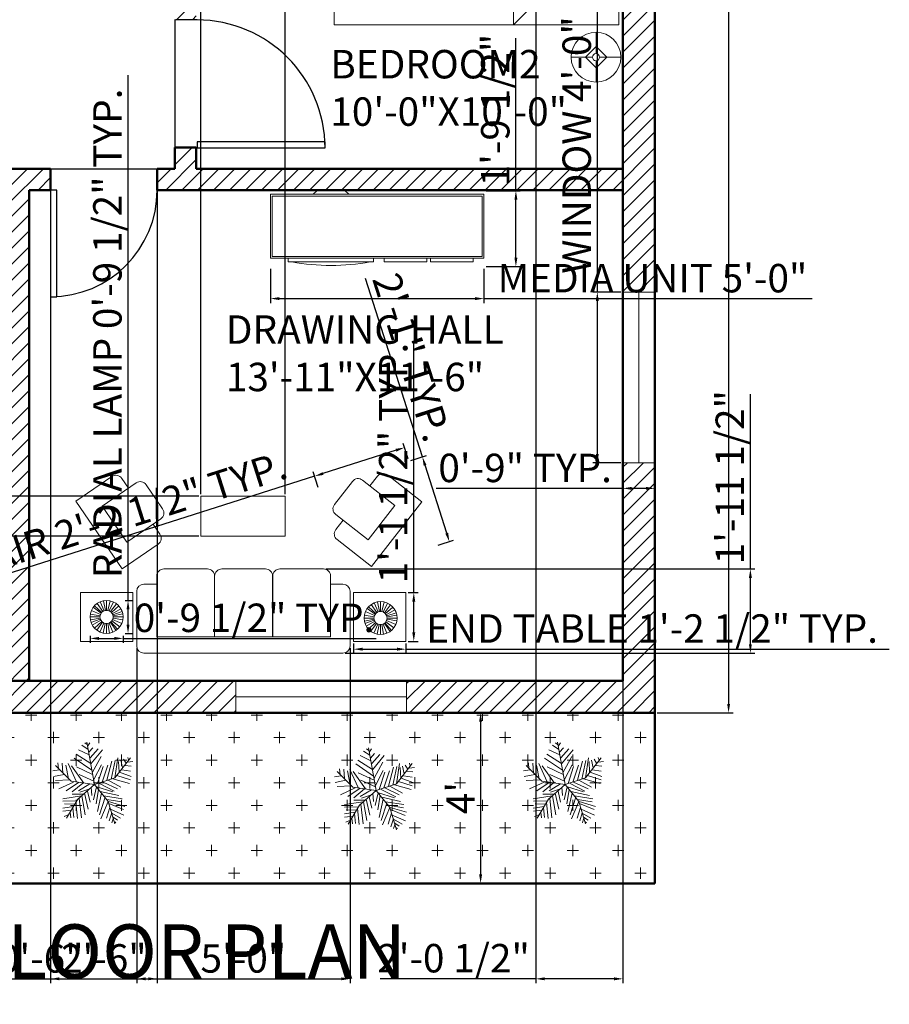
# Model space of a CAD drawing. Units: inches. Extents: x 1188 to 1681, y 1982 to 2608.
# Tile 2 of 4: x 1389 to 1634, y 1982 to 2259. Entities that reach past the tile are written whole.
import ezdxf

# ---------------------------------------------------------------- set-up
doc = ezdxf.new("R2010")
doc.units = ezdxf.units.IN
for name, color, linetype, lineweight in [('A-ANNO-DIMS', 2, 'Continuous', 18), ('A-ANNO-TEXT', 7, 'Continuous', 25), ('A-AREA-IDEN', 7, 'Continuous', 18), ('A-DOOR', 4, 'Continuous', 25), ('A-FURN', 8, 'Continuous', 18), ('A-GLAZ', 4, 'Continuous', 20), ('A-WALL', 7, 'Continuous', 50), ('A-WALL-PATT', 8, 'Continuous', 13)]:
    doc.layers.add(name, color=color, linetype=linetype, lineweight=lineweight)
doc.layers.add('L-PLNT', color=116, linetype='Continuous', lineweight=18, true_color=0x136734)
doc.layers.add('L-PLNT-PATT', color=116, linetype='Continuous', lineweight=13, true_color=0x136734)
doc.styles.get("Standard").update_dxf_attribs({"font": 'arial.ttf'})
doc.dimstyles.new('ISO-25', dxfattribs={"dimtxt": 8, "dimasz": 2.5, "dimexe": 1.25, "dimexo": 0.625, "dimtad": 1, "dimdec": 1, "dimlunit": 4, "dimtxsty": 'Standard', "dimcen": 2.5, "dimadec": 0, "dimazin": 0, "dimtfac": 1, "dimtdec": 1, "dimtmove": 0, "dimatfit": 3, "dimfxl": 1, "dimarcsym": 0})

# ---------------------------------------------------------------- blocks, each defined once
blk = doc.blocks.new('*U4')
for p, q in [((0, 0), (0, -6)), ((-36, 0), (-36, -6))]:
    blk.add_line(p, q)
blk.add_lwpolyline([(0, 0), (0, 36), (-1.75, 36), (-1.75, 0)], close=True)
blk.add_arc((0, 0), 36, 90, 180)
blk = doc.blocks.new('*U3')
for p, q in [((0, 0), (0, 6)), ((30, 0), (30, 6))]:
    blk.add_line(p, q)
blk.add_lwpolyline([(0, 0), (0, -30), (1.75, -30), (1.75, 0)], close=True)
blk.add_arc((0, 0), 30, 270, 0)
blk = doc.blocks.new('Entertainment Center')
for p, q in [((-4, 0), (-5, -1)), ((4, 0), (-4, 0)), ((5, -1), (4, 0)), ((-17, -19), (-17, -1)), ((-17, -1), (43, -1)), ((-16.5, -18.5), (-16.5, -1.5)), ((-16.5, -1.5), (42.5, -1.5)), ((42.5, -1.5), (42.5, -18.5)), ((43, -1), (43, -19)), ((43, -19), (-17, -19)), ((42.5, -18.5), (-16.5, -18.5)), ((-12, -20), (-12, -19)), ((12, -19), (12, -20)), ((15, -20), (15, -19)), ((27, -19), (27, -20)), ((28, -20), (28, -19)), ((40, -19), (40, -20)), ((12, -20), (-12, -20)), ((27, -20), (15, -20)), ((40, -20), (28, -20))]:
    blk.add_line(p, q)
blk.add_arc((0, 40), 61, 259.6111, 280.3889)
blk = doc.blocks.new('Lamp - Table')
for p, q in [((0, 7), (0, 1)), ((0, 3), (-3, 0)), ((3, 0), (0, 3)), ((-1, 0), (-7, 0)), ((-3, 0), (0, -3)), ((0, -3), (3, 0)), ((1, 0), (7, 0)), ((0, -1), (0, -7))]:
    blk.add_line(p, q)
for radius in [7, 1]:
    blk.add_circle((0, 0), radius)
blk = doc.blocks.new('Bed - Queen')
for p, q in [((0, -80.00003), (0, 0)), ((0, 0), (59.99999, 0)), ((59.99999, 0), (59.99999, -80.00003)), ((7.99999, -1.2), (28.79998, -1.2)), ((7.99999, -14.4), (7.99999, -1.2)), ((28.79998, -1.2), (28.79998, -14.4)), ((31.19999, -1.2), (51.99999, -1.2)), ((31.19999, -14.4), (31.19999, -1.2)), ((51.99999, -1.2), (51.99999, -16.4)), ((0, -14.4), (44.8, -14.4)), ((59.99999, -29.6), (44.8, -14.4)), ((44.8, -14.4), (44.8, -29.6)), ((51.99999, -16.4), (46.79936, -16.4)), ((44.8, -16.8), (0, -16.8)), ((44.8, -29.6), (59.99999, -29.6)), ((59.99999, -80.00003), (0, -80.00003))]:
    blk.add_line(p, q)
blk = doc.blocks.new('*U12')
for p, q in [((-8.737, 47.138), (-17.069, 52.711)), ((-10.186, 53.64), (-13.084, 55.962)), ((0, 0), (-10.5, 57)), ((-9.099, 51.782), (-6.563, 55.962)), ((-5.114, 28.097), (-24.676, 40.636)), ((-7.288, 39.707), (-21.778, 46.673)), ((-7.65, 43.423), (-2.578, 49.46)), ((-5.839, 35.992), (4.667, 48.067)), ((-5.114, 27.632), (10.463, 46.673)), ((-48.585, 21.131), (-49.309, 29.026)), ((-43.513, 28.561), (-42.427, 15.558)), ((-35.544, 28.097), (-24.314, 3.947)), ((-3.665, 19.273), (-27.574, 35.527)), ((-2.941, 16.486), (8.652, 37.85)), ((-1.129, 6.734), (9.014, 26.704)), ((16.259, 5.805), (23.142, 31.348)), ((22.055, 7.198), (27.489, 32.277)), ((27, 9), (48, 36)), ((27.127, 9.056), (31.112, 35.992)), ((31.836, 30.883), (32.561, 16.486)), ((35.096, 32.741), (37.27, 22.524)), ((38.719, 34.134), (41.979, 28.561)), ((43.791, 29.954), (51.036, 30.883)), ((44.153, 36.456), (45.239, 32.741)), ((-47.498, 19.737), (-55.83, 18.344)), ((-40.615, 13.7), (-55.105, 10.913)), ((-31.5, 4.5), (-52.5, 25.5)), ((-38.442, 26.239), (-34.819, 7.663)), ((-14.533, 2.09), (-30.834, 25.31)), ((-24.314, 23.917), (-2.941, 13.7)), ((-20.691, 13.7), (-1.129, 4.876)), ((3.942, 1.625), (11.187, 24.381)), ((10.101, 3.483), (17.708, 26.239)), ((33.285, 16.486), (48.862, 10.913)), ((36.183, 19.737), (48.137, 17.88)), ((40.53, 25.775), (48.862, 24.846)), ((-33.37, 6.269), (-52.207, 5.34)), ((-28.299, 3.483), (-47.86, -5.805)), ((-21.416, 3.018), (-38.079, -8.128)), ((0, 0), (-31.5, 4.5)), ((-15.982, 2.09), (-30.11, -9.521)), ((0, 0), (-22.5, -19.5)), ((-6.563, 1.161), (-21.416, -8.128)), ((0, 0), (27, 9)), ((0, 0), (18, -22.5)), ((6.478, 1.625), (26.04, -8.592)), ((11.187, 3.483), (30.749, -5.805)), ((18.07, 5.805), (35.096, -3.483)), ((24.229, 7.663), (46.688, 1.625)), ((29.662, 12.307), (48.137, 6.269)), ((-15.257, -12.772), (-30.11, -12.772)), ((-6.563, -5.805), (-19.967, -9.985)), ((-13.446, -11.378), (-8.737, -32.741)), ((-9.461, -8.592), (-6.201, -23.453)), ((-4.752, -3.483), (-3.665, -14.629)), ((2.493, -3.019), (-1.491, -20.202)), ((1.769, -2.555), (24.229, -9.521)), ((5.029, -6.27), (2.131, -25.775)), ((9.014, -11.378), (3.58, -35.992)), ((7.565, -9.056), (32.198, -14.629)), ((-17.431, -15.094), (-42.789, -18.809)), ((-24.314, -21.596), (-42.427, -22.06)), ((-26.849, -26.24), (-40.253, -25.775)), ((-22.5, -19.5), (-37.5, -45)), ((-25.038, -23.918), (-22.865, -45.281)), ((-20.691, -18.345), (-17.793, -44.352)), ((-17.069, -15.094), (-12.721, -40.172)), ((14.085, -16.951), (6.478, -40.172)), ((18.07, -22.524), (8.289, -45.745)), ((12.274, -15.094), (36.907, -18.809)), ((16.259, -19.738), (36.183, -22.989)), ((18, -22.5), (27, -52.5)), ((18.433, -22.524), (40.53, -29.026)), ((19.157, -25.311), (38.719, -33.206)), ((-28.299, -29.026), (-42.789, -31.348)), ((-30.834, -34.135), (-42.427, -35.528)), ((-32.646, -36.921), (-31.921, -44.352)), ((-29.023, -30.884), (-27.936, -43.887)), ((20.244, -30.419), (15.897, -44.816)), ((22.78, -37.85), (19.519, -48.532)), ((21.331, -32.741), (39.081, -40.636)), ((22.78, -38.314), (34.372, -44.816)), ((-34.457, -39.708), (-40.978, -42.494)), ((24.591, -45.745), (23.142, -50.854)), ((24.591, -43.423), (30.749, -47.603)), ((26.764, -49.925), (28.213, -50.854))]:
    blk.add_line(p, q)
blk = doc.blocks.new('*D13')
at = {"layer": 'A-ANNO-DIMS', "color": 0, "lineweight": -2, "transparency": 16777216}
for p, q in [((1568.34, 2496.41), (1589.68, 2496.41)), ((1588.43, 2493.91), (1588.43, 2066.91)), ((1568.34, 2064.41), (1589.68, 2064.41))]:
    blk.add_line(p, q, dxfattribs=at)
at = {"layer": 'A-ANNO-DIMS', "color": 0, "transparency": 16777216}
for points in [[(1588.02, 2493.91), (1588.85, 2493.91), (1588.43, 2496.41)], [(1588.02, 2066.91), (1588.85, 2066.91), (1588.43, 2064.41)]]:
    blk.add_solid(points, dxfattribs=at)
at = {"layer": 'Defpoints', "color": 0, "transparency": 16777216}
for p in [(1567.72, 2496.41), (1567.72, 2064.41), (1588.43, 2064.41)]:
    blk.add_point(p, dxfattribs=at)
at = {"layer": 'A-ANNO-DIMS', "color": 0, "transparency": 16777216, "insert": (1583.72, 2280.41), "char_height": 8, "attachment_point": 5, "rotation": 90}
blk.add_mtext("36'", dxfattribs=at)
blk = doc.blocks.new('*D15')
at = {"layer": 'A-ANNO-DIMS', "color": 0, "lineweight": -2, "transparency": 16777216}
for p, q in [((1512.39, 2064.41), (1519.94, 2064.41)), ((1518.69, 2061.91), (1518.69, 2018.91)), ((1512.39, 2016.41), (1519.94, 2016.41))]:
    blk.add_line(p, q, dxfattribs=at)
at = {"layer": 'A-ANNO-DIMS', "color": 0, "transparency": 16777216}
for points in [[(1518.27, 2061.91), (1519.1, 2061.91), (1518.69, 2064.41)], [(1518.27, 2018.91), (1519.1, 2018.91), (1518.69, 2016.41)]]:
    blk.add_solid(points, dxfattribs=at)
at = {"layer": 'Defpoints', "color": 0, "transparency": 16777216}
for p in [(1511.77, 2064.41), (1511.77, 2016.41), (1518.69, 2016.41)]:
    blk.add_point(p, dxfattribs=at)
at = {"layer": 'A-ANNO-DIMS', "color": 0, "transparency": 16777216, "insert": (1514.06, 2040.41), "char_height": 8, "attachment_point": 5, "rotation": 90}
blk.add_mtext("4'", dxfattribs=at)
blk = doc.blocks.new('WIN-48IN')
for p, q in [((0, 9), (0, 0)), ((48, 0), (48, 9)), ((48, 9), (48, 4.5)), ((48, 4.5), (0, 4.5)), ((0, 0), (48, 0))]:
    blk.add_line(p, q)
blk = doc.blocks.new('CHAIR-LOUNGE')
for p, q in [((10.14, 25.95), (0, 18.99)), ((14.8, 22.68), (12.92, 25.43)), ((0, 18.99), (13.03, 0)), ((23.68, 9.73), (21.74, 12.56)), ((13.03, 0), (23.17, 6.95))]:
    blk.add_line(p, q)
blk.add_lwpolyline([(16.97, 24.17), (7.41, 17.62), (14.35, 7.5), (23.91, 14.05, 0.414214), (24.43, 16.83), (19.75, 23.65, 0.414214)], format="xyb", close=True)
for centre, start, end in [((11.27, 24.3), 34.4415, 124.4415), ((22.03, 8.6), 304.4415, 34.4415)]:
    blk.add_arc(centre, 2, start, end)
blk = doc.blocks.new('LAMP-RADIAL-TABLE')
for p, q in [((1.97, 8.43), (3.57, 6.16)), ((3.57, 6.16), (1.97, 8.43)), ((3.92, 6.36), (2.86, 8.92)), ((2.86, 8.92), (3.92, 6.36)), ((4.31, 6.47), (3.81, 9.2)), ((3.81, 9.2), (4.31, 6.47)), ((4.64, 6.5), (4.64, 9.28)), ((5.01, 6.46), (5.61, 9.18)), ((5.61, 9.18), (5.03, 6.46)), ((5.41, 6.34), (6.55, 8.87)), ((5.75, 6.14), (7.4, 8.37)), ((7.4, 8.37), (5.75, 6.14)), ((2.93, 5.37), (0.37, 6.46)), ((0.89, 7.37), (3.13, 5.74)), ((3.13, 5.74), (0.89, 7.37)), ((3.28, 5.91), (1.25, 7.8)), ((6.03, 5.88), (8.1, 7.73)), ((6.26, 5.56), (8.67, 6.93)), ((8.67, 6.93), (6.26, 5.56)), ((6.4, 5.24), (9.03, 6.15)), ((2.78, 4.64), (0, 4.64)), ((0.07, 5.42), (2.8, 4.95)), ((2.8, 4.95), (0.07, 5.42)), ((2.8, 4.34), (0.08, 3.8)), ((0.08, 3.8), (2.81, 4.3)), ((2.88, 4.04), (0.25, 3.13)), ((0.25, 3.13), (2.88, 4.04)), ((0.6, 2.35), (3.02, 3.72)), ((3.02, 3.72), (0.6, 2.35)), ((3.26, 3.39), (1.21, 1.52)), ((1.88, 0.91), (3.52, 3.15)), ((3.53, 3.14), (1.88, 0.91)), ((3.87, 2.94), (2.73, 0.41)), ((3.67, 0.1), (4.23, 2.82)), ((4.25, 2.82), (3.67, 0.1)), ((4.64, 2.78), (4.64, 0)), ((5.47, 0.07), (4.97, 2.81)), ((4.97, 2.81), (5.47, 0.07)), ((5.36, 2.92), (6.42, 0.36)), ((7.31, 0.85), (5.71, 3.12)), ((5.71, 3.12), (7.31, 0.85)), ((5.88, 3.25), (7.72, 1.17)), ((6.14, 3.54), (8.39, 1.91)), ((8.39, 1.91), (6.14, 3.54)), ((6.35, 3.91), (8.91, 2.82)), ((8.91, 2.82), (6.35, 3.91)), ((6.47, 4.98), (9.2, 5.48)), ((9.21, 3.85), (6.47, 4.32)), ((6.47, 4.32), (9.21, 3.85)), ((9.28, 4.64), (6.5, 4.64))]:
    blk.add_line(p, q)
for radius in [4.64, 1.86]:
    blk.add_circle((4.64, 4.64), radius)
blk = doc.blocks.new('TABLE-END')
blk.add_lwpolyline([(14.72, 0), (0, 0), (0, 13.7), (14.72, 13.7)], close=True)
blk = doc.blocks.new('*D26')
at = {"layer": 'A-ANNO-DIMS', "color": 0, "lineweight": -2, "transparency": 16777216}
for p, q in [((1551.52, 2182.72), (1551.52, 2287.7)), ((1558.09, 2182.72), (1550.27, 2182.72)), ((1551.52, 2137.22), (1551.52, 2180.22)), ((1558.09, 2134.72), (1550.27, 2134.72))]:
    blk.add_line(p, q, dxfattribs=at)
at = {"layer": 'A-ANNO-DIMS', "color": 0, "transparency": 16777216}
for points in [[(1551.1, 2180.22), (1551.93, 2180.22), (1551.52, 2182.72)], [(1551.1, 2137.22), (1551.93, 2137.22), (1551.52, 2134.72)]]:
    blk.add_solid(points, dxfattribs=at)
at = {"layer": 'Defpoints', "color": 0, "transparency": 16777216}
for p in [(1551.52, 2182.72), (1558.72, 2182.72), (1558.72, 2134.72)]:
    blk.add_point(p, dxfattribs=at)
at = {"layer": 'A-ANNO-DIMS', "color": 0, "transparency": 16777216, "insert": (1546.75, 2236.46), "char_height": 8, "attachment_point": 5, "rotation": 90}
blk.add_mtext('WINDOW 4\'-0" TYP.', dxfattribs=at)
blk = doc.blocks.new('*D27')
at = {"layer": 'A-ANNO-DIMS', "color": 0, "lineweight": -2, "transparency": 16777216}
for p, q in [((1558.72, 2134.09), (1558.72, 2126.27)), ((1567.72, 2134.09), (1567.72, 2126.27)), ((1558.72, 2127.52), (1506.2, 2127.52)), ((1565.22, 2127.52), (1561.22, 2127.52))]:
    blk.add_line(p, q, dxfattribs=at)
at = {"layer": 'A-ANNO-DIMS', "color": 0, "transparency": 16777216}
for points in [[(1561.22, 2127.93), (1561.22, 2127.1), (1558.72, 2127.52)], [(1565.22, 2127.93), (1565.22, 2127.1), (1567.72, 2127.52)]]:
    blk.add_solid(points, dxfattribs=at)
at = {"layer": 'Defpoints', "color": 0, "transparency": 16777216}
for p in [(1558.72, 2134.72), (1567.72, 2134.72), (1558.72, 2127.52)]:
    blk.add_point(p, dxfattribs=at)
at = {"layer": 'A-ANNO-DIMS', "color": 0, "transparency": 16777216, "insert": (1531.21, 2132.23), "char_height": 8, "attachment_point": 5}
blk.add_mtext('0\'-9" TYP.', dxfattribs=at)
blk = doc.blocks.new('*D30')
at = {"layer": 'A-ANNO-DIMS', "color": 0, "lineweight": -2, "transparency": 16777216}
for p, q in [((1494.92, 2138.23), (1474.36, 2131.69)), ((1498.32, 2135.79), (1496.92, 2140.18)), ((1471.98, 2130.93), (1320.5, 2082.67)), ((1473, 2127.73), (1471.6, 2132.12))]:
    blk.add_line(p, q, dxfattribs=at)
at = {"layer": 'A-ANNO-DIMS', "color": 0, "transparency": 16777216}
for points in [[(1494.79, 2138.63), (1495.04, 2137.84), (1497.3, 2138.99)], [(1474.24, 2132.08), (1474.49, 2131.29), (1471.98, 2130.93)]]:
    blk.add_solid(points, dxfattribs=at)
at = {"layer": 'Defpoints', "color": 0, "transparency": 16777216}
for p in [(1498.51, 2135.2), (1471.98, 2130.93), (1473.19, 2127.13)]:
    blk.add_point(p, dxfattribs=at)
at = {"layer": 'A-ANNO-DIMS', "color": 0, "transparency": 16777216, "insert": (1393.6, 2110.96), "char_height": 8, "attachment_point": 5, "rotation": 17.6695}
blk.add_mtext('LOUNGE CHAIR 2\'-2 1/2" TYP.', dxfattribs=at)
blk = doc.blocks.new('*D31')
at = {"layer": 'A-ANNO-DIMS', "color": 0, "lineweight": -2, "transparency": 16777216}
for p, q in [((1502.31, 2136.41), (1486.33, 2186.57)), ((1499.1, 2135.39), (1503.5, 2136.79)), ((1509.15, 2114.91), (1503.07, 2134.02)), ((1506.71, 2111.51), (1511.1, 2112.91))]:
    blk.add_line(p, q, dxfattribs=at)
at = {"layer": 'A-ANNO-DIMS', "color": 0, "transparency": 16777216}
for points in [[(1503.46, 2134.15), (1502.67, 2133.9), (1502.31, 2136.41)], [(1509.55, 2115.04), (1508.76, 2114.79), (1509.91, 2112.53)]]:
    blk.add_solid(points, dxfattribs=at)
at = {"layer": 'Defpoints', "color": 0, "transparency": 16777216}
for p in [(1502.31, 2136.41), (1498.51, 2135.2), (1506.11, 2111.32)]:
    blk.add_point(p, dxfattribs=at)
at = {"layer": 'A-ANNO-DIMS', "color": 0, "transparency": 16777216, "insert": (1498.36, 2164.09), "char_height": 8, "attachment_point": 5, "rotation": 287.6695}
blk.add_mtext('2\'-1" TYP.', dxfattribs=at)
blk = doc.blocks.new('*D32')
at = {"layer": 'A-ANNO-DIMS', "color": 0, "lineweight": -2, "transparency": 16777216}
for p, q in [((1419.52, 2095.98), (1419.52, 2243.74)), ((1418.76, 2095.98), (1420.77, 2095.98)), ((1419.52, 2089.2), (1419.52, 2093.48)), ((1418.76, 2086.7), (1420.77, 2086.7))]:
    blk.add_line(p, q, dxfattribs=at)
at = {"layer": 'A-ANNO-DIMS', "color": 0, "transparency": 16777216}
for points in [[(1419.11, 2093.48), (1419.94, 2093.48), (1419.52, 2095.98)], [(1419.11, 2089.2), (1419.94, 2089.2), (1419.52, 2086.7)]]:
    blk.add_solid(points, dxfattribs=at)
at = {"layer": 'Defpoints', "color": 0, "transparency": 16777216}
for p in [(1418.13, 2095.98), (1419.52, 2095.98), (1418.13, 2086.7)]:
    blk.add_point(p, dxfattribs=at)
at = {"layer": 'A-ANNO-DIMS', "color": 0, "transparency": 16777216, "insert": (1414.76, 2171.11), "char_height": 8, "attachment_point": 5, "rotation": 90}
blk.add_mtext('RADIAL LAMP 0\'-9 1/2" TYP.', dxfattribs=at)
blk = doc.blocks.new('*D33')
at = {"layer": 'A-ANNO-DIMS', "color": 0, "lineweight": -2, "transparency": 16777216}
for p, q in [((1408.85, 2086.08), (1408.85, 2084.06)), ((1418.13, 2086.08), (1418.13, 2084.06)), ((1411.35, 2085.31), (1415.63, 2085.31)), ((1418.13, 2085.31), (1489.29, 2085.31))]:
    blk.add_line(p, q, dxfattribs=at)
at = {"layer": 'A-ANNO-DIMS', "color": 0, "transparency": 16777216}
for points in [[(1411.35, 2085.73), (1411.35, 2084.89), (1408.85, 2085.31)], [(1415.63, 2085.73), (1415.63, 2084.89), (1418.13, 2085.31)]]:
    blk.add_solid(points, dxfattribs=at)
at = {"layer": 'Defpoints', "color": 0, "transparency": 16777216}
for p in [(1408.85, 2086.7), (1418.13, 2086.7), (1418.13, 2085.31)]:
    blk.add_point(p, dxfattribs=at)
at = {"layer": 'A-ANNO-DIMS', "color": 0, "transparency": 16777216, "insert": (1454.96, 2090.07), "char_height": 8, "attachment_point": 5}
blk.add_mtext('0\'-9 1/2" TYP.', dxfattribs=at)
blk = doc.blocks.new('*D34')
at = {"layer": 'A-ANNO-DIMS', "color": 0, "lineweight": -2, "transparency": 16777216}
for p, q in [((1482.97, 2083.87), (1482.97, 2081.03)), ((1497.69, 2083.87), (1497.69, 2081.03)), ((1485.47, 2082.28), (1495.19, 2082.28)), ((1497.69, 2082.28), (1633.64, 2082.28))]:
    blk.add_line(p, q, dxfattribs=at)
at = {"layer": 'A-ANNO-DIMS', "color": 0, "transparency": 16777216}
for points in [[(1485.47, 2082.7), (1485.47, 2081.87), (1482.97, 2082.28)], [(1495.19, 2082.7), (1495.19, 2081.87), (1497.69, 2082.28)]]:
    blk.add_solid(points, dxfattribs=at)
at = {"layer": 'Defpoints', "color": 0, "transparency": 16777216}
for p in [(1482.97, 2084.49), (1497.69, 2084.49), (1497.69, 2082.28)]:
    blk.add_point(p, dxfattribs=at)
at = {"layer": 'A-ANNO-DIMS', "color": 0, "transparency": 16777216, "insert": (1566.91, 2087.05), "char_height": 8, "attachment_point": 5}
blk.add_mtext('END TABLE 1\'-2 1/2" TYP.', dxfattribs=at)
blk = doc.blocks.new('*D35')
at = {"layer": 'A-ANNO-DIMS', "color": 0, "lineweight": -2, "transparency": 16777216}
for p, q in [((1499.9, 2098.19), (1499.9, 2168.6)), ((1498.31, 2098.19), (1501.15, 2098.19)), ((1499.9, 2086.99), (1499.9, 2095.69)), ((1498.31, 2084.49), (1501.15, 2084.49))]:
    blk.add_line(p, q, dxfattribs=at)
at = {"layer": 'A-ANNO-DIMS', "color": 0, "transparency": 16777216}
for points in [[(1499.48, 2095.69), (1500.31, 2095.69), (1499.9, 2098.19)], [(1499.48, 2086.99), (1500.31, 2086.99), (1499.9, 2084.49)]]:
    blk.add_solid(points, dxfattribs=at)
at = {"layer": 'Defpoints', "color": 0, "transparency": 16777216}
for p in [(1497.69, 2098.19), (1499.9, 2098.19), (1497.69, 2084.49)]:
    blk.add_point(p, dxfattribs=at)
at = {"layer": 'A-ANNO-DIMS', "color": 0, "transparency": 16777216, "insert": (1495.14, 2134.64), "char_height": 8, "attachment_point": 5, "rotation": 90}
blk.add_mtext('1\'-1 1/2" TYP.', dxfattribs=at)
blk = doc.blocks.new('*D40')
at = {"layer": 'A-ANNO-DIMS', "color": 0, "lineweight": -2, "transparency": 16777216}
for p, q in [((1459.61, 2189.27), (1459.61, 2179.64)), ((1519.61, 2189.27), (1519.61, 2179.64)), ((1462.11, 2180.89), (1517.11, 2180.89)), ((1519.61, 2180.89), (1611.94, 2180.89))]:
    blk.add_line(p, q, dxfattribs=at)
at = {"layer": 'A-ANNO-DIMS', "color": 0, "transparency": 16777216}
for points in [[(1462.11, 2181.31), (1462.11, 2180.47), (1459.61, 2180.89)], [(1517.11, 2181.31), (1517.11, 2180.47), (1519.61, 2180.89)]]:
    blk.add_solid(points, dxfattribs=at)
at = {"layer": 'Defpoints', "color": 0, "transparency": 16777216}
for p in [(1459.61, 2189.89), (1519.61, 2189.89), (1519.61, 2180.89)]:
    blk.add_point(p, dxfattribs=at)
at = {"layer": 'A-ANNO-DIMS', "color": 0, "transparency": 16777216, "insert": (1567.03, 2185.6), "char_height": 8, "attachment_point": 5}
blk.add_mtext('MEDIA UNIT 5\'-0"', dxfattribs=at)
blk = doc.blocks.new('*D41')
at = {"layer": 'A-ANNO-DIMS', "color": 0, "lineweight": -2, "transparency": 16777216}
for p, q in [((1528.61, 2211.22), (1528.61, 2254.13)), ((1520.24, 2211.22), (1529.86, 2211.22)), ((1528.61, 2192.39), (1528.61, 2208.72)), ((1520.24, 2189.89), (1529.86, 2189.89))]:
    blk.add_line(p, q, dxfattribs=at)
at = {"layer": 'A-ANNO-DIMS', "color": 0, "transparency": 16777216}
for points in [[(1528.2, 2208.72), (1529.03, 2208.72), (1528.61, 2211.22)], [(1528.2, 2192.39), (1529.03, 2192.39), (1528.61, 2189.89)]]:
    blk.add_solid(points, dxfattribs=at)
at = {"layer": 'Defpoints', "color": 0, "transparency": 16777216}
for p in [(1519.61, 2211.22), (1528.61, 2211.22), (1519.61, 2189.89)]:
    blk.add_point(p, dxfattribs=at)
at = {"layer": 'A-ANNO-DIMS', "color": 0, "transparency": 16777216, "insert": (1523.85, 2233.93), "char_height": 8, "attachment_point": 5, "rotation": 90}
blk.add_mtext('1\'-9 1/2"', dxfattribs=at)
blk = doc.blocks.new('*D48')
at = {"layer": 'A-ANNO-DIMS', "color": 0, "lineweight": -2, "transparency": 16777216}
for p, q in [((1397.72, 2216.79), (1397.72, 1988.31)), ((1427.72, 2216.79), (1427.72, 1988.31)), ((1400.22, 1989.56), (1425.22, 1989.56))]:
    blk.add_line(p, q, dxfattribs=at)
at = {"layer": 'A-ANNO-DIMS', "color": 0, "transparency": 16777216}
for points in [[(1400.22, 1989.98), (1400.22, 1989.15), (1397.72, 1989.56)], [(1425.22, 1989.98), (1425.22, 1989.15), (1427.72, 1989.56)]]:
    blk.add_solid(points, dxfattribs=at)
at = {"layer": 'Defpoints', "color": 0, "transparency": 16777216}
for p in [(1397.72, 2217.41), (1427.72, 2217.41), (1427.72, 1989.56)]:
    blk.add_point(p, dxfattribs=at)
at = {"layer": 'A-ANNO-DIMS', "color": 0, "transparency": 16777216, "insert": (1412.72, 1994.27), "char_height": 8, "attachment_point": 5}
blk.add_mtext('2\'-6"', dxfattribs=at)
blk = doc.blocks.new('*D50')
at = {"layer": 'A-ANNO-DIMS', "color": 0, "lineweight": -2, "transparency": 16777216}
for p, q in [((1372.72, 2342.79), (1372.72, 1988.31)), ((1378.72, 2336.79), (1378.72, 1988.31)), ((1370.22, 1989.56), (1367.72, 1989.56)), ((1372.72, 1989.56), (1378.72, 1989.56)), ((1381.22, 1989.56), (1406.23, 1989.56))]:
    blk.add_line(p, q, dxfattribs=at)
at = {"layer": 'A-ANNO-DIMS', "color": 0, "transparency": 16777216}
for points in [[(1370.22, 1989.98), (1370.22, 1989.15), (1372.72, 1989.56)], [(1381.22, 1989.98), (1381.22, 1989.15), (1378.72, 1989.56)]]:
    blk.add_solid(points, dxfattribs=at)
at = {"layer": 'Defpoints', "color": 0, "transparency": 16777216}
for p in [(1372.72, 2343.41), (1378.72, 2337.41), (1378.72, 1989.56)]:
    blk.add_point(p, dxfattribs=at)
at = {"layer": 'A-ANNO-DIMS', "color": 0, "transparency": 16777216, "insert": (1394.97, 1994.27), "char_height": 8, "attachment_point": 5}
blk.add_mtext('0\'-6"', dxfattribs=at)
blk = doc.blocks.new('*D52')
at = {"layer": 'A-ANNO-DIMS', "color": 0, "lineweight": -2, "transparency": 16777216}
for p, q in [((1534.2, 2391.18), (1534.2, 1988.31)), ((1558.72, 2391.18), (1558.72, 1988.31)), ((1534.2, 1989.56), (1490.41, 1989.56)), ((1556.22, 1989.56), (1536.7, 1989.56))]:
    blk.add_line(p, q, dxfattribs=at)
at = {"layer": 'A-ANNO-DIMS', "color": 0, "transparency": 16777216}
for points in [[(1536.7, 1989.98), (1536.7, 1989.15), (1534.2, 1989.56)], [(1556.22, 1989.98), (1556.22, 1989.15), (1558.72, 1989.56)]]:
    blk.add_solid(points, dxfattribs=at)
at = {"layer": 'Defpoints', "color": 0, "transparency": 16777216}
for p in [(1534.2, 2391.81), (1558.72, 2391.81), (1534.2, 1989.56)]:
    blk.add_point(p, dxfattribs=at)
at = {"layer": 'A-ANNO-DIMS', "color": 0, "transparency": 16777216, "insert": (1511.06, 1994.33), "char_height": 8, "attachment_point": 5}
blk.add_mtext('2\'-0 1/2"', dxfattribs=at)
blk = doc.blocks.new('*D57')
at = {"layer": 'A-ANNO-DIMS', "color": 0, "lineweight": -2, "transparency": 16777216}
for p, q in [((1440.02, 2125.93), (1440.02, 2524.51)), ((1442.52, 2523.26), (1461.18, 2523.26)), ((1463.68, 2125.93), (1463.68, 2524.51)), ((1463.68, 2523.26), (1512.8, 2523.26))]:
    blk.add_line(p, q, dxfattribs=at)
at = {"layer": 'A-ANNO-DIMS', "color": 0, "transparency": 16777216}
for points in [[(1442.52, 2523.68), (1442.52, 2522.85), (1440.02, 2523.26)], [(1461.18, 2523.68), (1461.18, 2522.85), (1463.68, 2523.26)]]:
    blk.add_solid(points, dxfattribs=at)
at = {"layer": 'Defpoints', "color": 0, "transparency": 16777216}
for p in [(1463.68, 2523.26), (1440.02, 2125.31), (1463.68, 2125.31)]:
    blk.add_point(p, dxfattribs=at)
at = {"layer": 'A-ANNO-DIMS', "color": 0, "transparency": 16777216, "insert": (1489.49, 2528.03), "char_height": 8, "attachment_point": 5}
blk.add_mtext('1\'-11 1/2"', dxfattribs=at)
blk = doc.blocks.new('*D58')
at = {"layer": 'A-ANNO-DIMS', "color": 0, "lineweight": -2, "transparency": 16777216}
for p, q in [((1204.87, 2125.31), (1204.87, 2175.18)), ((1439.4, 2125.31), (1203.62, 2125.31)), ((1204.87, 2116.54), (1204.87, 2122.81)), ((1439.4, 2114.04), (1203.62, 2114.04))]:
    blk.add_line(p, q, dxfattribs=at)
at = {"layer": 'A-ANNO-DIMS', "color": 0, "transparency": 16777216}
for points in [[(1204.45, 2122.81), (1205.28, 2122.81), (1204.87, 2125.31)], [(1204.45, 2116.54), (1205.28, 2116.54), (1204.87, 2114.04)]]:
    blk.add_solid(points, dxfattribs=at)
at = {"layer": 'Defpoints', "color": 0, "transparency": 16777216}
for p in [(1204.87, 2125.31), (1440.02, 2125.31), (1440.02, 2114.04)]:
    blk.add_point(p, dxfattribs=at)
at = {"layer": 'A-ANNO-DIMS', "color": 0, "transparency": 16777216, "insert": (1200.11, 2151.49), "char_height": 8, "attachment_point": 5, "rotation": 90}
blk.add_mtext('0\'-11 1/2"', dxfattribs=at)
blk = doc.blocks.new('*D59')
at = {"layer": 'A-ANNO-DIMS', "color": 0, "lineweight": -2, "transparency": 16777216}
for p, q in [((1421.97, 2082.56), (1421.97, 1988.31)), ((1481.97, 2082.56), (1481.97, 1988.31)), ((1424.47, 1989.56), (1479.47, 1989.56))]:
    blk.add_line(p, q, dxfattribs=at)
at = {"layer": 'A-ANNO-DIMS', "color": 0, "transparency": 16777216}
for points in [[(1424.47, 1989.98), (1424.47, 1989.15), (1421.97, 1989.56)], [(1479.47, 1989.98), (1479.47, 1989.15), (1481.97, 1989.56)]]:
    blk.add_solid(points, dxfattribs=at)
at = {"layer": 'Defpoints', "color": 0, "transparency": 16777216}
for p in [(1421.97, 2083.18), (1481.97, 2083.18), (1481.97, 1989.56)]:
    blk.add_point(p, dxfattribs=at)
at = {"layer": 'A-ANNO-DIMS', "color": 0, "transparency": 16777216, "insert": (1451.97, 1994.27), "char_height": 8, "attachment_point": 5}
blk.add_mtext('5\'-0"', dxfattribs=at)
blk = doc.blocks.new('*D60')
at = {"layer": 'A-ANNO-DIMS', "color": 0, "lineweight": -2, "transparency": 16777216}
for p, q in [((1594.57, 2104.85), (1594.57, 2153.97)), ((1475.13, 2104.85), (1595.82, 2104.85)), ((1594.57, 2083.68), (1594.57, 2102.35)), ((1480.59, 2081.18), (1595.82, 2081.18))]:
    blk.add_line(p, q, dxfattribs=at)
at = {"layer": 'A-ANNO-DIMS', "color": 0, "transparency": 16777216}
for points in [[(1594.15, 2102.35), (1594.98, 2102.35), (1594.57, 2104.85)], [(1594.15, 2083.68), (1594.98, 2083.68), (1594.57, 2081.18)]]:
    blk.add_solid(points, dxfattribs=at)
at = {"layer": 'Defpoints', "color": 0, "transparency": 16777216}
for p in [(1474.51, 2104.85), (1594.57, 2104.85), (1479.97, 2081.18)]:
    blk.add_point(p, dxfattribs=at)
at = {"layer": 'A-ANNO-DIMS', "color": 0, "transparency": 16777216, "insert": (1589.81, 2130.66), "char_height": 8, "attachment_point": 5, "rotation": 90}
blk.add_mtext('1\'-11 1/2"', dxfattribs=at)

msp = doc.modelspace()

# ---------------------------------------------------------------- hatches: boundary and pattern name
at = {"layer": 'A-WALL-PATT', "transparency": 33554559}
h = msp.add_hatch(dxfattribs=at)
h.set_pattern_fill('ANSI31', color=256)
h.paths.add_polyline_path([(1390.99, 2496.41), (1231.72, 2496.41), (1231.72, 2452.82), (1240.72, 2452.82), (1240.72, 2487.41), (1390.99, 2487.41)])
h.paths.add_polyline_path([(1469.3, 2496.41), (1426.99, 2496.41), (1426.99, 2491.91), (1426.99, 2487.41), (1469.3, 2487.41)])
h.paths.add_polyline_path([(1378.72, 2487.41), (1372.72, 2487.41), (1372.72, 2404.84), (1372.72, 2343.41), (1367.48, 2343.41), (1367.48, 2337.41), (1378.72, 2337.41), (1378.72, 2391.41), (1387.67, 2391.41), (1387.67, 2397.41), (1378.72, 2397.41)])
h.paths.add_polyline_path([(1438.72, 2487.41), (1432.72, 2487.41), (1432.72, 2397.41), (1420.72, 2397.41), (1420.72, 2391.41), (1432.72, 2391.41), (1432.72, 2385.41), (1438.72, 2385.41)])
h.paths.add_polyline_path([(1240.72, 2392.82), (1236.22, 2392.82), (1231.72, 2392.82), (1231.72, 2323.77), (1240.72, 2323.77)])
h.paths.add_polyline_path([(1330.72, 2343.41), (1240.72, 2343.41), (1240.72, 2337.41), (1330.72, 2337.41)])
h.paths.add_polyline_path([(1558.72, 2343.41), (1438.72, 2343.41), (1438.72, 2349.29), (1438.64, 2349.29), (1432.72, 2349.29), (1432.72, 2259.41), (1438.72, 2259.41), (1438.72, 2337.41), (1558.72, 2337.41)])
h.paths.add_polyline_path([(1567.72, 2396.81), (1558.72, 2396.81), (1558.72, 2317.68), (1563.22, 2317.68), (1567.72, 2317.68)])
h.paths.add_polyline_path([(1567.72, 2496.41), (1529.3, 2496.41), (1529.3, 2491.91), (1529.3, 2487.41), (1558.72, 2487.41), (1558.72, 2461.81), (1567.72, 2461.81)])
h.paths.add_polyline_path([(1240.72, 2195.41), (1240.72, 2201.41), (1240.72, 2263.77), (1231.72, 2263.77), (1231.72, 2016.41), (1246.72, 2016.41), (1246.72, 2022.41), (1246.72, 2025.41), (1240.72, 2025.41)])
h.paths.add_polyline_path([(1391.72, 2211.41), (1397.72, 2211.41), (1397.72, 2217.41), (1385.72, 2217.41), (1385.72, 2163.41), (1366.72, 2163.41), (1366.72, 2157.41), (1385.72, 2157.41), (1385.72, 2073.41), (1391.72, 2073.41)])
h.paths.add_polyline_path([(1330.72, 2201.41), (1282.72, 2201.41), (1282.72, 2195.41), (1324.72, 2195.41), (1324.72, 2064.41), (1345.75, 2064.41), (1345.75, 2073.41), (1330.72, 2073.41), (1330.72, 2157.41), (1336.72, 2157.41), (1336.72, 2163.41), (1330.72, 2163.41)])
h.paths.add_polyline_path([(1558.72, 2217.41), (1438.72, 2217.41), (1438.72, 2223.26), (1432.72, 2223.26), (1432.72, 2217.41), (1427.72, 2217.41), (1427.72, 2211.41), (1432.72, 2211.41), (1558.72, 2211.41)])
h.paths.add_polyline_path([(1567.72, 2269.68), (1558.72, 2269.68), (1558.72, 2182.72), (1563.22, 2182.72), (1567.72, 2182.72)])
h.paths.add_polyline_path([(1567.72, 2134.72), (1558.72, 2134.72), (1558.72, 2073.41), (1497.85, 2073.41), (1497.85, 2068.91), (1497.85, 2064.41), (1567.72, 2064.41)])
h.paths.add_polyline_path([(1449.85, 2073.41), (1371.31, 2073.41), (1371.31, 2068.91), (1371.31, 2064.41), (1449.85, 2064.41)])
h.paths.add_polyline_path([(1333.72, 2064.41), (1324.72, 2064.41), (1324.72, 2025.41), (1313.9, 2025.41), (1313.9, 2016.41), (1333.72, 2016.41)])
at = {"layer": 'L-PLNT-PATT', "transparency": 33554679}
h = msp.add_hatch(dxfattribs=at)
h.set_pattern_fill('CROSS', color=256)
h.paths.add_polyline_path([(1567.72, 2064.41), (1333.72, 2064.41), (1333.72, 2016.41), (1567.72, 2016.41)])

# ---------------------------------------------------------------- linework, layer by layer
at = {"layer": 'A-DOOR'}
for p, q in [((1432.72, 2259.41), (1432.72, 2223.41)), ((1397.72, 2217.41), (1427.72, 2217.41))]:
    msp.add_line(p, q, dxfattribs=at)
at = {"layer": 'A-FURN'}
for p, q in [((1427.59, 2100.56), (1423.97, 2100.56)), ((1479.97, 2100.56), (1476.51, 2100.56)), ((1421.97, 2098.56), (1421.97, 2083.18)), ((1481.97, 2083.18), (1481.97, 2098.56)), ((1423.97, 2081.18), (1479.97, 2081.18))]:
    msp.add_line(p, q, dxfattribs=at)
msp.add_lwpolyline([(1440.02, 2114.04), (1463.68, 2114.04), (1463.68, 2125.31), (1440.02, 2125.31)], close=True, dxfattribs=at)
for points in [[(1429.59, 2104.85), (1441.86, 2104.85, -0.414214), (1443.86, 2102.85), (1443.86, 2085.8), (1427.59, 2085.8), (1427.59, 2102.85, -0.414214)], [(1445.89, 2104.85), (1458.17, 2104.85, -0.414214), (1460.17, 2102.85), (1460.17, 2085.8), (1443.89, 2085.8), (1443.89, 2102.85, -0.414214)], [(1462.23, 2104.85), (1474.51, 2104.85, -0.414214), (1476.51, 2102.85), (1476.51, 2085.8), (1460.23, 2085.8), (1460.23, 2102.85, -0.414214)]]:
    msp.add_lwpolyline(points, format="xyb", close=True, dxfattribs=at)
for centre, start, end in [((1423.97, 2098.56), 90, 180), ((1479.97, 2098.56), 0, 90), ((1423.97, 2083.18), 180, 270), ((1479.97, 2083.18), 270, 0)]:
    msp.add_arc(centre, 2, start, end, dxfattribs=at)
at = {"layer": 'A-WALL'}
for p, q in [((1567.72, 2496.41), (1567.72, 2016.41)), ((1558.72, 2487.41), (1558.72, 2073.41)), ((1432.72, 2223.41), (1438.72, 2223.41)), ((1432.72, 2223.41), (1432.72, 2217.41)), ((1438.72, 2223.41), (1438.72, 2217.41)), ((1385.72, 2217.41), (1397.72, 2217.41)), ((1397.72, 2217.41), (1397.72, 2211.41)), ((1427.72, 2217.41), (1427.72, 2211.41)), ((1427.72, 2217.41), (1432.72, 2217.41)), ((1438.72, 2217.41), (1558.72, 2217.41)), ((1391.72, 2211.41), (1391.72, 2073.41)), ((1391.72, 2211.41), (1397.72, 2211.41)), ((1427.72, 2211.41), (1432.72, 2211.41)), ((1432.72, 2211.41), (1558.72, 2211.41)), ((1330.72, 2073.41), (1558.72, 2073.41)), ((1324.72, 2064.41), (1567.72, 2064.41)), ((1282.72, 2016.41), (1567.72, 2016.41))]:
    msp.add_line(p, q, dxfattribs=at)

# ---------------------------------------------------------------- block references
at = {"layer": 'A-DOOR', "rotation": 270}
msp.add_blockref('*U4', (1438.93, 2223.26), dxfattribs=at)
at = {"layer": 'A-DOOR'}
msp.add_blockref('*U3', (1397.72, 2211.41), dxfattribs=at)
at = {"layer": 'A-FURN'}
for name, p, rotation in [('Bed - Queen', (1557.52, 2317.86), 270), ('CHAIR-LOUNGE', (1506.11, 2111.32), 107.669519136369)]:
    msp.add_blockref(name, p, dxfattribs=dict(at, rotation=rotation))
for name, p in [('Lamp - Table', (1551.15, 2248.79)), ('Entertainment Center', (1476.61, 2211.22)), ('CHAIR-LOUNGE', (1404.83, 2104.89)), ('TABLE-END', (1406.13, 2084.49)), ('TABLE-END', (1482.97, 2084.49)), ('LAMP-RADIAL-TABLE', (1408.85, 2086.7)), ('LAMP-RADIAL-TABLE', (1485.91, 2086.4))]:
    msp.add_blockref(name, p, dxfattribs=at)
at = {"layer": 'A-GLAZ', "rotation": 89.99999999999909}
msp.add_blockref('WIN-48IN', (1567.72, 2134.72), dxfattribs=at)
at = {"layer": 'A-GLAZ'}
msp.add_blockref('WIN-48IN', (1449.85, 2064.41), dxfattribs=at)
at = {"layer": 'L-PLNT', "xscale": 0.2102822374520575, "yscale": 0.2102822374520575, "zscale": 0.2102822374520575}
for p in [(1410.14, 2044.18), (1542.5, 2044.18), (1489.36, 2042.52)]:
    msp.add_blockref('*U12', p, dxfattribs=at)

# ---------------------------------------------------------------- texts
at = {"layer": 'A-ANNO-TEXT', "insert": (1281.99, 2004.88), "char_height": 15.2538, "attachment_point": 1}
msp.add_mtext_dynamic_manual_height_columns('GROUND FLOOR PLAN', width=268.1014, gutter_width=23.83, heights=[0], dxfattribs=at)
at = {"layer": 'A-AREA-IDEN', "char_height": 8, "attachment_point": 1}
for s, insert in [('BEDROOM2\\P10\'-0"X10\'-0"', (1476.41, 2250.82)), ('DRAWING HALL\\P13\'-11"X11\'-6"', (1447.03, 2176.18))]:
    msp.add_mtext(s, dxfattribs=dict(at, insert=insert))

# ---------------------------------------------------------------- dimensions: what is measured, and where the dimension line sits
at = {"layer": 'A-ANNO-DIMS'}
for base, p1, p2, picture, middle in [((1463.68, 2523.26), (1440.02, 2125.31), (1463.68, 2125.31), '*D57', (1489.49, 2528.03)), ((1534.2, 1989.56), (1558.72, 2391.81), (1534.2, 2391.81), '*D52', (1511.06, 1994.33)), ((1378.72, 1989.56), (1372.72, 2343.41), (1378.72, 2337.41), '*D50', (1394.97, 1994.27)), ((1427.72, 1989.56), (1397.72, 2217.41), (1427.72, 2217.41), '*D48', (1412.72, 1994.27)), ((1481.97, 1989.56), (1421.97, 2083.18), (1481.97, 2083.18), '*D59', (1451.97, 1994.27))]:
    dim = msp.add_linear_dim(base=base, p1=p1, p2=p2, dimstyle='ISO-25', override={"dimdec": 1, "dimlfac": 1, "dimrnd": 0, "dimzin": 1, "dimdsep": 46, "dimlunit": 4, "dimfrac": 2}, dxfattribs=at)
    dim.commit()
    dim.dimension.update_dxf_attribs({"geometry": picture, "text_midpoint": middle})
for base, p1, p2, override, picture, middle in [((1588.43, 2064.41), (1567.72, 2496.41), (1567.72, 2064.41), {"dimclrd": 0, "dimclre": 0, "dimclrt": 0}, '*D13', (1583.72, 2280.41)), ((1528.61, 2211.22), (1519.61, 2189.89), (1519.61, 2211.22), {"dimdec": 1, "dimlfac": 1, "dimrnd": 0, "dimzin": 1, "dimdsep": 46, "dimlunit": 4, "dimfrac": 2}, '*D41', (1523.85, 2233.93)), ((1204.87, 2125.31), (1440.02, 2114.04), (1440.02, 2125.31), {"dimdec": 1, "dimlfac": 1, "dimrnd": 0, "dimzin": 1, "dimdsep": 46, "dimlunit": 4, "dimfrac": 2}, '*D58', (1200.11, 2151.49)), ((1594.57, 2104.85), (1479.97, 2081.18), (1474.51, 2104.85), {"dimdec": 1, "dimlfac": 1, "dimrnd": 0, "dimzin": 1, "dimdsep": 46, "dimlunit": 4, "dimfrac": 2}, '*D60', (1589.81, 2130.66)), ((1518.69, 2016.41), (1511.77, 2064.41), (1511.77, 2016.41), {"dimclrd": 0, "dimclre": 0, "dimclrt": 0}, '*D15', (1514.06, 2040.41))]:
    dim = msp.add_linear_dim(base=base, p1=p1, p2=p2, angle=90, dimstyle='ISO-25', override=override, dxfattribs=at)
    dim.commit()
    dim.dimension.update_dxf_attribs({"geometry": picture, "text_midpoint": middle})
for base, p1, p2, angle, text, picture, middle in [((1551.52, 2182.72), (1558.72, 2134.72), (1558.72, 2182.72), 90, 'WINDOW <> TYP.', '*D26', (1546.75, 2236.46)), ((1419.52, 2095.98), (1418.13, 2086.7), (1418.13, 2095.98), 90, 'RADIAL LAMP <> TYP.', '*D32', (1414.76, 2171.11)), ((1502.31, 2136.41), (1506.11, 2111.32), (1498.51, 2135.2), 107.6695, '<> TYP.', '*D31', (1498.36, 2164.09)), ((1499.9, 2098.19), (1497.69, 2084.49), (1497.69, 2098.19), 90, '<> TYP.', '*D35', (1495.14, 2134.64)), ((1471.98, 2130.93), (1498.51, 2135.2), (1473.19, 2127.13), 197.6695, 'LOUNGE CHAIR <> TYP.', '*D30', (1393.6, 2110.96)), ((1558.72, 2127.52), (1567.72, 2134.72), (1558.72, 2134.72), 180, '<> TYP.', '*D27', (1531.21, 2132.23))]:
    dim = msp.add_linear_dim(base=base, p1=p1, p2=p2, angle=angle, text=text, dimstyle='ISO-25', override={"dimdec": 1, "dimlfac": 1, "dimrnd": 0, "dimzin": 1, "dimdsep": 46, "dimlunit": 4, "dimfrac": 2}, dxfattribs=at)
    dim.commit()
    dim.dimension.update_dxf_attribs({"geometry": picture, "text_midpoint": middle})
for base, p1, p2, text, picture, middle in [((1519.61, 2180.89), (1459.61, 2189.89), (1519.61, 2189.89), 'MEDIA UNIT <>', '*D40', (1567.03, 2185.6)), ((1497.69, 2082.28), (1482.97, 2084.49), (1497.69, 2084.49), 'END TABLE <> TYP.', '*D34', (1566.91, 2087.05)), ((1418.13, 2085.31), (1408.85, 2086.7), (1418.13, 2086.7), '<> TYP.', '*D33', (1454.96, 2090.07))]:
    dim = msp.add_linear_dim(base=base, p1=p1, p2=p2, text=text, dimstyle='ISO-25', override={"dimdec": 1, "dimlfac": 1, "dimrnd": 0, "dimzin": 1, "dimdsep": 46, "dimlunit": 4, "dimfrac": 2}, dxfattribs=at)
    dim.commit()
    dim.dimension.update_dxf_attribs({"geometry": picture, "text_midpoint": middle})

doc.saveas('drawing.dxf')
